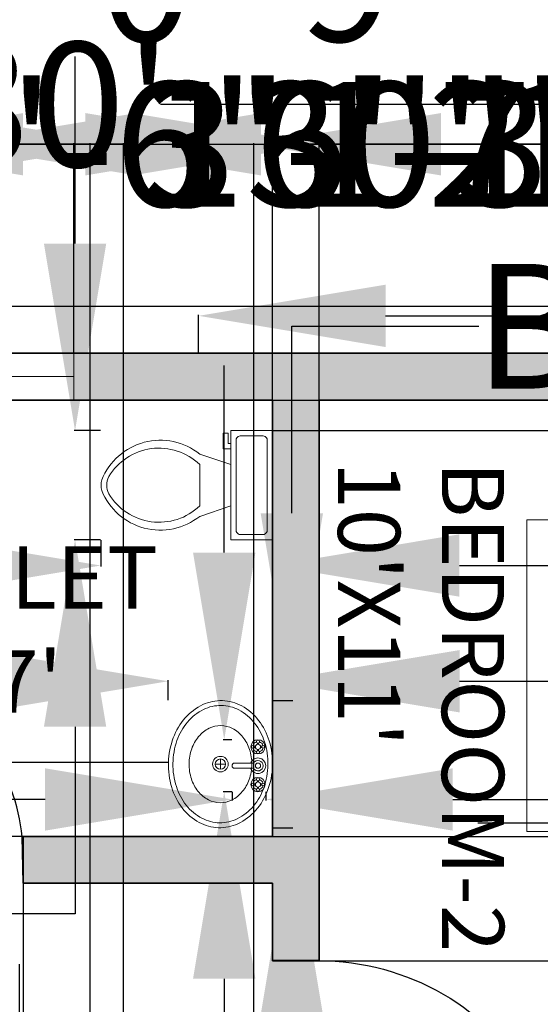
# Model space of a CAD drawing. Units: inches. Extents: x 2838 to 4029, y 1041 to 1915.
# Tile 12 of 16: x 3441 to 3541, y 1546 to 1735. Entities that reach past the tile are written whole.
import ezdxf

# ---------------------------------------------------------------- set-up
doc = ezdxf.new("R2010")
doc.units = ezdxf.units.IN
doc.header["$MEASUREMENT"] = 0
for name, color, linetype, lineweight in [('A-ANNO-DIMS', 2, 'Continuous', 18), ('A-AREA-IDEN', 7, 'Continuous', 18), ('A-DOOR', 3, 'Continuous', 25), ('A-FLOR', 7, 'Continuous', 25), ('A-FLOR-FIXT', 9, 'Continuous', 18), ('A-FURN', 8, 'Continuous', 18), ('A-GLAZ', 4, 'Continuous', 18), ('A-WALL', 7, 'Continuous', 35), ('A-WALL-PATT', 252, 'Continuous', 13)]:
    doc.layers.add(name, color=color, linetype=linetype, lineweight=lineweight)
doc.styles.get("Standard").update_dxf_attribs({"font": 'arial.ttf'})
doc.dimstyles.get("Standard").update_dxf_attribs({"dimtxt": 24, "dimasz": 36, "dimexe": 0.18, "dimexo": 0.0625, "dimgap": 0.09, "dimtad": 0, "dimtih": 1, "dimtoh": 1, "dimdec": 0, "dimzin": 0, "dimdsep": 46, "dimlunit": 3, "dimtxsty": 'Standard', "dimcen": 0.09, "dimadec": 0, "dimazin": 0, "dimtfac": 1, "dimtdec": 0, "dimtofl": 0, "dimtmove": 0, "dimatfit": 3, "dimfxl": 1, "dimtolj": 1, "dimtzin": 0, "dimarcsym": 0})

# ---------------------------------------------------------------- blocks, each defined once
blk = doc.blocks.new('*U2')
for p, q in [((0, 0), (0, -6)), ((40, 0), (40, -6))]:
    blk.add_line(p, q)
blk.add_lwpolyline([(0, 0), (34.64, 20), (35.52, 18.48), (0.87, -1.52)], close=True)
blk.add_arc((0, 0), 40, 0, 30)
blk = doc.blocks.new('*U3')
for p, q in [((-40, 0), (-40, 6)), ((0, 0), (0, 6))]:
    blk.add_line(p, q)
blk.add_lwpolyline([(0, 0), (-20, -34.64), (-21.52, -33.77), (-1.52, 0.88)], close=True)
blk.add_arc((0, 0), 40, 180, 240)
blk = doc.blocks.new('Toilet - top')
for p, q in [((9.5, -6), (9.5, -2)), ((-10, -8.5), (-8, -8.5)), ((-10, -9.5), (-10, -8.5)), ((-8, -8.5), (-8, -8)), ((-7, -8), (-7, -9.5)), ((-4, -8), (-6, -14)), ((4, -8), (6, -14)), ((-7, -9.5), (-10, -9.5)), ((4, -14), (-4, -14))]:
    blk.add_line(p, q)
blk.add_lwpolyline([(10.5, -8), (10.5, 0), (-10.5, 0), (-10.5, -8)], close=True)
for points in [[(8.5, -1), (-8.5, -1)], [(-9.5, -2), (-9.5, -6)], [(-8.5, -7), (8.5, -7)]]:
    blk.add_lwpolyline(points)
for centre, radius, start, end in [((-8.62, -1.88), 0.884, 81.8699, 188.1301), ((8.62, -1.88), 0.884, 351.8699, 98.1301), ((-8.62, -6.12), 0.884, 171.8699, 278.1301), ((8.62, -6.12), 0.884, 261.8699, 8.1301), ((3.52, -21.58), 12.17, 141.4691, 247.9714), ((4.2, -21.82), 11.33, 136.3677, 238.9468), ((-3.52, -21.58), 12.17, 292.0284, 38.5307), ((-4.2, -21.82), 11.33, 301.053, 43.6321), ((0, -27.88), 4, 245.7318, 294.2682), ((0, -29), 4, 254.8605, 285.1395)]:
    blk.add_arc(centre, radius, start, end)
blk = doc.blocks.new('Sink - Oval top')
for p, q in [((-1, 0), (1, 0)), ((0, 1), (0, -1))]:
    blk.add_line(p, q)
for points in [[(-12.23, 0.39, 0.117634), (-11.46, -3.36, 0.104469), (-8.88, -6.8, 0.090016), (-5.08, -9.07, 0.08192), (-0.32, -10.02, 0.08192), (4.49, -9.38, 0.090016), (8.42, -7.36, 0.104469), (11.22, -4.09, 0.117634), (12.23, -0.39, 0.117634), (11.46, 3.36, 0.104469), (8.88, 6.8, 0.090016), (5.08, 9.07, 0.08192), (0.32, 10.02, 0.08192), (-4.49, 9.38, 0.090016), (-8.42, 7.36, 0.104469), (-11.22, 4.09, 0.117634)], [(-11.29, 0.16, 0.118622), (-10.52, -3.25, 0.104678), (-8.07, -6.36, 0.089562), (-4.54, -8.37, 0.081185), (-0.13, -9.15, 0.081185), (4.3, -8.49, 0.089562), (7.89, -6.58, 0.104678), (10.42, -3.55, 0.118622), (11.29, -0.16, 0.118622), (10.52, 3.25, 0.104678), (8.07, 6.36, 0.089562), (4.54, 8.37, 0.081185), (0.13, 9.15, 0.081185), (-4.3, 8.49, 0.089562), (-7.89, 6.58, 0.104678), (-10.42, 3.55, 0.118622)], [(-7.42, 0.08, 0.118283), (-6.91, -2.17, 0.104607), (-5.29, -4.21, 0.089718), (-2.97, -5.53, 0.081436), (-0.07, -6.04, 0.081436), (2.84, -5.59, 0.089718), (5.2, -4.33, 0.104607), (6.86, -2.32, 0.118283), (7.42, -0.08, 0.118283), (6.91, 2.17, 0.104607), (5.29, 4.21, 0.089718), (2.97, 5.53, 0.081436), (0.07, 6.04, 0.081436), (-2.84, 5.59, 0.089718), (-5.2, 4.33, 0.104607), (-6.86, 2.32, 0.118283)]]:
    blk.add_lwpolyline(points, format="xyb", close=True)
for radius in [1.5, 1]:
    blk.add_circle((0, 0), radius)
blk = doc.blocks.new('Bed - Queen')
for p, q in [((0, -80.00003), (0, 0)), ((0, 0), (59.99999, 0)), ((59.99999, 0), (59.99999, -80.00003)), ((7.99999, -1.2), (28.79998, -1.2)), ((7.99999, -14.4), (7.99999, -1.2)), ((28.79998, -1.2), (28.79998, -14.4)), ((31.19999, -1.2), (51.99999, -1.2)), ((31.19999, -14.4), (31.19999, -1.2)), ((51.99999, -1.2), (51.99999, -16.4)), ((0, -14.4), (44.8, -14.4)), ((59.99999, -29.6), (44.8, -14.4)), ((44.8, -14.4), (44.8, -29.6)), ((44.8, -16.8), (0, -16.8)), ((51.99999, -16.4), (46.79936, -16.4)), ((44.8, -29.6), (59.99999, -29.6)), ((59.99999, -80.00003), (0, -80.00003))]:
    blk.add_line(p, q)
blk = doc.blocks.new('Faucet - Bathroom top')
for p, q in [((-4.107, 0.125), (-4.375, 0.125)), ((-3.75, 0.4788), (-3.75, 0.75)), ((-3.5, 0.482), (-3.5, 0.75)), ((-3.1461, 0.125), (-2.875, 0.125)), ((3.143, 0.125), (2.875, 0.125)), ((3.5, 0.4788), (3.5, 0.75)), ((3.75, 0.482), (3.75, 0.75)), ((4.1039, 0.125), (4.375, 0.125)), ((-4.1039, -0.125), (-4.375, -0.125)), ((-3.75, -0.4821), (-3.75, -0.75)), ((-3.5, -0.4789), (-3.5, -0.75)), ((-3.143, -0.125), (-2.875, -0.125)), ((-0.5, -0.8639), (-0.5, -4.5)), ((0.5, -4.5), (0.5, -0.8631)), ((3.1461, -0.125), (2.875, -0.125)), ((3.5, -0.4821), (3.5, -0.75)), ((3.75, -0.4789), (3.75, -0.75)), ((4.107, -0.125), (4.375, -0.125))]:
    blk.add_line(p, q)
for centre, radius in [((-3.625, 0), 1.375), ((-4.625, 0), 0.2795), ((-3.625, 0), 0.5), ((-3.625, 1), 0.2795), ((-2.625, 0), 0.2795), ((0, 0), 0.5), ((3.625, 0), 1.375), ((2.625, 0), 0.2795), ((3.625, 0), 0.5), ((3.625, 1), 0.2795), ((4.625, 0), 0.2795), ((-3.625, -1), 0.2795), ((3.625, -1), 0.2795)]:
    blk.add_circle(centre, radius)
for centre, radius, start, end in [((-3.625, 0), 1, 105.2407, 164.2093), ((-3.625, 0), 1, 16.44125, 74.07887), ((0, 0), 1.5, 289.6514, 250.3603), ((0, 0), 1, 300.3431, 239.7554), ((3.625, 0), 1, 106.12, 164.0884), ((3.625, 0), 1, 16.23422, 73.90469), ((-3.625, 0), 1, 196.2342, 253.9047), ((-3.625, 0), 1, 286.12, 344.0884), ((3.625, 0), 1, 196.4413, 254.0789), ((3.625, 0), 1, 285.2407, 344.2093), ((0, -4.5), 0.5, 180, 0)]:
    blk.add_arc(centre, radius, start, end)
blk = doc.blocks.new('*D18')
at = {"layer": 'A-ANNO-DIMS', "color": 0, "lineweight": -2, "transparency": 16777216}
for p, q in [((3267.73, 1671.36), (3267.73, 1719.35)), ((3303.73, 1719.17), (3427.28, 1719.17)), ((3591.73, 1719.17), (3468.18, 1719.17)), ((3627.73, 1671.36), (3627.73, 1719.35))]:
    blk.add_line(p, q, dxfattribs=at)
at = {"layer": 'A-ANNO-DIMS', "color": 0, "transparency": 16777216}
for points in [[(3303.73, 1725.17), (3303.73, 1713.17), (3267.73, 1719.17)], [(3591.73, 1725.17), (3591.73, 1713.17), (3627.73, 1719.17)]]:
    blk.add_solid(points, dxfattribs=at)
at = {"layer": 'Defpoints', "color": 0, "transparency": 16777216}
for p in [(3267.73, 1719.17), (3267.73, 1671.3), (3627.73, 1671.3)]:
    blk.add_point(p, dxfattribs=at)
at = {"layer": 'A-ANNO-DIMS', "color": 0, "transparency": 16777216, "insert": (3447.73, 1719.17), "char_height": 24, "attachment_point": 5}
blk.add_mtext("\\A1;30'", dxfattribs=at)
blk = doc.blocks.new('WIN-24-VENT')
for p, q in [((24, 9), (24, 0)), ((24, 4.5), (0, 4.5))]:
    blk.add_line(p, q)
blk.add_lwpolyline([(48, 0), (0, 0), (0, 9), (48, 9)])
blk = doc.blocks.new('*D28')
at = {"layer": 'A-ANNO-DIMS', "color": 0, "lineweight": -2, "transparency": 16777216}
for p, q in [((3565.25, 1580.88), (3529.25, 1580.88)), ((3601.25, 1578.37), (3601.25, 1581.06)), ((3617.82, 1578.37), (3617.82, 1581.06)), ((3653.82, 1580.88), (3689.82, 1580.88))]:
    blk.add_line(p, q, dxfattribs=at)
at = {"layer": 'A-ANNO-DIMS', "color": 0, "transparency": 16777216}
for points in [[(3565.25, 1586.88), (3565.25, 1574.88), (3601.25, 1580.88)], [(3653.82, 1586.88), (3653.82, 1574.88), (3617.82, 1580.88)]]:
    blk.add_solid(points, dxfattribs=at)
at = {"layer": 'Defpoints', "color": 0, "transparency": 16777216}
for p in [(3617.82, 1580.88), (3601.25, 1578.31), (3617.82, 1578.31)]:
    blk.add_point(p, dxfattribs=at)
at = {"layer": 'A-ANNO-DIMS', "color": 0, "transparency": 16777216, "insert": (3789.89, 1580.88), "char_height": 24, "attachment_point": 5}
blk.add_mtext('\\A1;1\'-4 1/2" TYP.', dxfattribs=at)
blk = doc.blocks.new('*D35')
at = {"layer": 'A-ANNO-DIMS', "color": 0, "lineweight": -2, "transparency": 16777216}
for p, q in [((3480.45, 1632.93), (3480.45, 1668.93)), ((3481.89, 1596.93), (3480.27, 1596.93)), ((3481.89, 1586.93), (3480.27, 1586.93)), ((3480.45, 1550.93), (3480.45, 1514.93)), ((3480.45, 1514.93), (3444.45, 1514.93))]:
    blk.add_line(p, q, dxfattribs=at)
at = {"layer": 'A-ANNO-DIMS', "color": 0, "transparency": 16777216}
for points in [[(3474.45, 1632.93), (3486.45, 1632.93), (3480.45, 1596.93)], [(3474.45, 1550.93), (3486.45, 1550.93), (3480.45, 1586.93)]]:
    blk.add_solid(points, dxfattribs=at)
at = {"layer": 'Defpoints', "color": 0, "transparency": 16777216}
for p in [(3481.95, 1596.93), (3480.45, 1586.93), (3481.95, 1586.93)]:
    blk.add_point(p, dxfattribs=at)
at = {"layer": 'A-ANNO-DIMS', "color": 0, "transparency": 16777216, "insert": (3365.58, 1514.93), "char_height": 24, "attachment_point": 5}
blk.add_mtext('\\A1;TAP 0\'-10"', dxfattribs=at)
blk = doc.blocks.new('*D36')
at = {"layer": 'A-ANNO-DIMS', "color": 0, "lineweight": -2, "transparency": 16777216}
for p, q in [((3481.95, 1586.87), (3481.95, 1585.25)), ((3488.45, 1586.87), (3488.45, 1585.25)), ((3445.95, 1585.43), (3409.95, 1585.43)), ((3524.45, 1585.43), (3560.45, 1585.43))]:
    blk.add_line(p, q, dxfattribs=at)
at = {"layer": 'A-ANNO-DIMS', "color": 0, "transparency": 16777216}
for points in [[(3445.95, 1591.43), (3445.95, 1579.43), (3481.95, 1585.43)], [(3524.45, 1591.43), (3524.45, 1579.43), (3488.45, 1585.43)]]:
    blk.add_solid(points, dxfattribs=at)
at = {"layer": 'Defpoints', "color": 0, "transparency": 16777216}
for p in [(3481.95, 1586.93), (3488.45, 1586.93), (3488.45, 1585.43)]:
    blk.add_point(p, dxfattribs=at)
at = {"layer": 'A-ANNO-DIMS', "color": 0, "transparency": 16777216, "insert": (3620.4, 1585.43), "char_height": 24, "attachment_point": 5}
blk.add_mtext('\\A1;0\'-6 1/2"', dxfattribs=at)
blk = doc.blocks.new('*D39')
at = {"layer": 'A-ANNO-DIMS', "color": 0, "lineweight": -2, "transparency": 16777216}
for p, q in [((3391.52, 1678.5), (3355.52, 1678.5)), ((3427.52, 1671.36), (3427.52, 1678.68)), ((3475.52, 1671.36), (3475.52, 1678.68)), ((3511.52, 1678.5), (3547.52, 1678.5))]:
    blk.add_line(p, q, dxfattribs=at)
at = {"layer": 'A-ANNO-DIMS', "color": 0, "transparency": 16777216}
for points in [[(3391.52, 1684.5), (3391.52, 1672.5), (3427.52, 1678.5)], [(3511.52, 1684.5), (3511.52, 1672.5), (3475.52, 1678.5)]]:
    blk.add_solid(points, dxfattribs=at)
at = {"layer": 'Defpoints', "color": 0, "transparency": 16777216}
for p in [(3475.52, 1678.5), (3427.52, 1671.3), (3475.52, 1671.3)]:
    blk.add_point(p, dxfattribs=at)
at = {"layer": 'A-ANNO-DIMS', "color": 0, "transparency": 16777216, "insert": (3732.24, 1678.5), "char_height": 24, "attachment_point": 5}
blk.add_mtext('\\A1;VENT BLOCK 4\'-0" TYP.', dxfattribs=at)
blk = doc.blocks.new('*D40')
at = {"layer": 'A-ANNO-DIMS', "color": 0, "lineweight": -2, "transparency": 16777216}
for p, q in [((3420.32, 1707.3), (3420.32, 1743.3)), ((3420.32, 1743.3), (3456.32, 1743.3)), ((3427.46, 1671.3), (3420.14, 1671.3)), ((3427.46, 1662.3), (3420.14, 1662.3)), ((3420.32, 1626.3), (3420.32, 1590.3))]:
    blk.add_line(p, q, dxfattribs=at)
at = {"layer": 'A-ANNO-DIMS', "color": 0, "transparency": 16777216}
for points in [[(3414.32, 1707.3), (3426.32, 1707.3), (3420.32, 1671.3)], [(3414.32, 1626.3), (3426.32, 1626.3), (3420.32, 1662.3)]]:
    blk.add_solid(points, dxfattribs=at)
at = {"layer": 'Defpoints', "color": 0, "transparency": 16777216}
for p in [(3420.32, 1671.3), (3427.52, 1671.3), (3427.52, 1662.3)]:
    blk.add_point(p, dxfattribs=at)
at = {"layer": 'A-ANNO-DIMS', "color": 0, "transparency": 16777216, "insert": (3529.56, 1743.3), "char_height": 24, "attachment_point": 5}
blk.add_mtext('\\A1;0\'-9" TYP.', dxfattribs=at)
blk = doc.blocks.new('*D41')
at = {"layer": 'A-ANNO-DIMS', "color": 0, "lineweight": -2, "transparency": 16777216}
for p, q in [((3284.24, 1506.2), (3284.24, 1496.56)), ((3347.73, 1506.2), (3347.73, 1496.56)), ((3248.24, 1496.74), (3212.24, 1496.74)), ((3383.73, 1496.74), (3419.73, 1496.74))]:
    blk.add_line(p, q, dxfattribs=at)
at = {"layer": 'A-ANNO-DIMS', "color": 0, "transparency": 16777216}
for points in [[(3248.24, 1502.74), (3248.24, 1490.74), (3284.24, 1496.74)], [(3383.73, 1502.74), (3383.73, 1490.74), (3347.73, 1496.74)]]:
    blk.add_solid(points, dxfattribs=at)
at = {"layer": 'Defpoints', "color": 0, "transparency": 16777216}
for p in [(3284.24, 1506.26), (3347.73, 1506.26), (3347.73, 1496.74)]:
    blk.add_point(p, dxfattribs=at)
at = {"layer": 'A-ANNO-DIMS', "color": 0, "transparency": 16777216, "insert": (3624.81, 1496.74), "char_height": 24, "attachment_point": 5}
blk.add_mtext('\\A1;WARDROBE 5\'-3 1/2" TYP.', dxfattribs=at)
blk = doc.blocks.new('*D45')
at = {"layer": 'A-ANNO-DIMS', "color": 0, "lineweight": -2, "transparency": 16777216}
for p, q in [((3456.69, 1635.35), (3456.69, 1630.27)), ((3489.73, 1635.35), (3489.73, 1630.27)), ((3420.69, 1630.45), (3384.69, 1630.45)), ((3525.73, 1630.45), (3561.73, 1630.45))]:
    blk.add_line(p, q, dxfattribs=at)
at = {"layer": 'A-ANNO-DIMS', "color": 0, "transparency": 16777216}
for points in [[(3420.69, 1636.45), (3420.69, 1624.45), (3456.69, 1630.45)], [(3525.73, 1636.45), (3525.73, 1624.45), (3489.73, 1630.45)]]:
    blk.add_solid(points, dxfattribs=at)
at = {"layer": 'Defpoints', "color": 0, "transparency": 16777216}
for p in [(3456.69, 1635.41), (3489.73, 1635.41), (3489.73, 1630.45)]:
    blk.add_point(p, dxfattribs=at)
at = {"layer": 'A-ANNO-DIMS', "color": 0, "transparency": 16777216, "insert": (3626.8, 1630.45), "char_height": 24, "attachment_point": 5}
blk.add_mtext('\\A1;WC 2\'-9"', dxfattribs=at)
blk = doc.blocks.new('*D46')
at = {"layer": 'A-ANNO-DIMS', "color": 0, "lineweight": -2, "transparency": 16777216}
for p, q in [((3451.73, 1692.41), (3451.73, 1728.41)), ((3456.62, 1656.41), (3451.55, 1656.41)), ((3456.62, 1635.41), (3451.55, 1635.41)), ((3451.73, 1599.41), (3451.73, 1563.41)), ((3451.73, 1563.41), (3415.73, 1563.41))]:
    blk.add_line(p, q, dxfattribs=at)
at = {"layer": 'A-ANNO-DIMS', "color": 0, "transparency": 16777216}
for points in [[(3445.73, 1692.41), (3457.73, 1692.41), (3451.73, 1656.41)], [(3445.73, 1599.41), (3457.73, 1599.41), (3451.73, 1635.41)]]:
    blk.add_solid(points, dxfattribs=at)
at = {"layer": 'Defpoints', "color": 0, "transparency": 16777216}
for p in [(3456.69, 1656.41), (3451.73, 1635.41), (3456.69, 1635.41)]:
    blk.add_point(p, dxfattribs=at)
at = {"layer": 'A-ANNO-DIMS', "color": 0, "transparency": 16777216, "insert": (3384.87, 1563.41), "char_height": 24, "attachment_point": 5}
blk.add_mtext('\\A1;1\'-9"', dxfattribs=at)
blk = doc.blocks.new('*D47')
at = {"layer": 'A-ANNO-DIMS', "color": 0, "lineweight": -2, "transparency": 16777216}
for p, q in [((3493.47, 1640.5), (3493.47, 1676.5)), ((3493.47, 1676.5), (3529.47, 1676.5)), ((3489.85, 1604.5), (3493.65, 1604.5)), ((3489.85, 1579.95), (3493.65, 1579.95)), ((3493.47, 1543.95), (3493.47, 1507.95))]:
    blk.add_line(p, q, dxfattribs=at)
at = {"layer": 'A-ANNO-DIMS', "color": 0, "transparency": 16777216}
for points in [[(3487.47, 1640.5), (3499.47, 1640.5), (3493.47, 1604.5)], [(3487.47, 1543.95), (3499.47, 1543.95), (3493.47, 1579.95)]]:
    blk.add_solid(points, dxfattribs=at)
at = {"layer": 'Defpoints', "color": 0, "transparency": 16777216}
for p in [(3489.78, 1604.5), (3493.47, 1604.5), (3489.78, 1579.95)]:
    blk.add_point(p, dxfattribs=at)
at = {"layer": 'A-ANNO-DIMS', "color": 0, "transparency": 16777216, "insert": (3643.85, 1676.5), "char_height": 24, "attachment_point": 5}
blk.add_mtext('\\A1;BASIN 2\'-0 1/2"', dxfattribs=at)
blk = doc.blocks.new('*D48')
at = {"layer": 'A-ANNO-DIMS', "color": 0, "lineweight": -2, "transparency": 16777216}
for p, q in [((3433.65, 1608.18), (3397.65, 1608.18)), ((3469.65, 1604.56), (3469.65, 1608.36)), ((3489.78, 1604.56), (3489.78, 1608.36)), ((3525.78, 1608.18), (3561.78, 1608.18))]:
    blk.add_line(p, q, dxfattribs=at)
at = {"layer": 'A-ANNO-DIMS', "color": 0, "transparency": 16777216}
for points in [[(3433.65, 1614.18), (3433.65, 1602.18), (3469.65, 1608.18)], [(3525.78, 1614.18), (3525.78, 1602.18), (3489.78, 1608.18)]]:
    blk.add_solid(points, dxfattribs=at)
at = {"layer": 'Defpoints', "color": 0, "transparency": 16777216}
for p in [(3469.65, 1608.18), (3469.65, 1604.5), (3489.78, 1604.5)]:
    blk.add_point(p, dxfattribs=at)
at = {"layer": 'A-ANNO-DIMS', "color": 0, "transparency": 16777216, "insert": (3366.79, 1608.18), "char_height": 24, "attachment_point": 5}
blk.add_mtext('\\A1;1\'-8"', dxfattribs=at)
blk = doc.blocks.new('*D50')
at = {"layer": 'A-ANNO-DIMS', "color": 0, "lineweight": -2, "transparency": 16777216}
for p, q in [((3441.02, 1517.75), (3441.02, 1553.75)), ((3427.44, 1481.75), (3441.2, 1481.75)), ((3427.44, 1426.75), (3441.2, 1426.75)), ((3441.02, 1390.75), (3441.02, 1354.75))]:
    blk.add_line(p, q, dxfattribs=at)
at = {"layer": 'A-ANNO-DIMS', "color": 0, "transparency": 16777216}
for points in [[(3435.02, 1517.75), (3447.02, 1517.75), (3441.02, 1481.75)], [(3435.02, 1390.75), (3447.02, 1390.75), (3441.02, 1426.75)]]:
    blk.add_solid(points, dxfattribs=at)
at = {"layer": 'Defpoints', "color": 0, "transparency": 16777216}
for p in [(3427.37, 1481.75), (3441.02, 1481.75), (3427.37, 1426.75)]:
    blk.add_point(p, dxfattribs=at)
at = {"layer": 'A-ANNO-DIMS', "color": 0, "transparency": 16777216, "insert": (3441.02, 1454.25), "char_height": 24, "attachment_point": 5}
blk.add_mtext('\\A1;4\'-7"', dxfattribs=at)
blk = doc.blocks.new('*D55')
at = {"layer": 'A-ANNO-DIMS', "color": 0, "lineweight": -2, "transparency": 16777216}
for p, q in [((3491.76, 1499.78), (3455.76, 1499.78)), ((3527.76, 1494.67), (3527.76, 1499.96)), ((3562.26, 1494.67), (3562.26, 1499.96)), ((3598.26, 1499.78), (3634.26, 1499.78))]:
    blk.add_line(p, q, dxfattribs=at)
at = {"layer": 'A-ANNO-DIMS', "color": 0, "transparency": 16777216}
for points in [[(3491.76, 1505.78), (3491.76, 1493.78), (3527.76, 1499.78)], [(3598.26, 1505.78), (3598.26, 1493.78), (3562.26, 1499.78)]]:
    blk.add_solid(points, dxfattribs=at)
at = {"layer": 'Defpoints', "color": 0, "transparency": 16777216}
for p in [(3527.76, 1499.78), (3527.76, 1494.6), (3562.26, 1494.6)]:
    blk.add_point(p, dxfattribs=at)
at = {"layer": 'A-ANNO-DIMS', "color": 0, "transparency": 16777216, "insert": (3260.33, 1499.78), "char_height": 24, "attachment_point": 5}
blk.add_mtext('\\A1;BASE CABINET 2\'-10 1/2"', dxfattribs=at)
blk = doc.blocks.new('*D68')
at = {"layer": 'A-ANNO-DIMS', "color": 0, "lineweight": -2, "transparency": 16777216}
for p, q in [((3258.73, 1680.36), (3258.73, 1711.7)), ((3294.73, 1711.52), (3406.43, 1711.52)), ((3600.73, 1711.52), (3489.04, 1711.52)), ((3636.73, 1680.36), (3636.73, 1711.7))]:
    blk.add_line(p, q, dxfattribs=at)
at = {"layer": 'A-ANNO-DIMS', "color": 0, "transparency": 16777216}
for points in [[(3294.73, 1717.52), (3294.73, 1705.52), (3258.73, 1711.52)], [(3600.73, 1717.52), (3600.73, 1705.52), (3636.73, 1711.52)]]:
    blk.add_solid(points, dxfattribs=at)
at = {"layer": 'Defpoints', "color": 0, "transparency": 16777216}
for p in [(3636.73, 1711.52), (3258.73, 1680.3), (3636.73, 1680.3)]:
    blk.add_point(p, dxfattribs=at)
at = {"layer": 'A-ANNO-DIMS', "color": 0, "transparency": 16777216, "insert": (3447.73, 1711.52), "char_height": 24, "attachment_point": 5}
blk.add_mtext('\\A1;31\'-6"', dxfattribs=at)
blk = doc.blocks.new('*D73')
at = {"layer": 'A-ANNO-DIMS', "color": 0, "lineweight": -2, "transparency": 16777216}
for p, q in [((3425.038746, 1711.522346), (3389.038746, 1711.522346)), ((3461.038746, 1200.359846), (3461.038746, 1711.702346)), ((3618.731626, 1200.359846), (3618.731626, 1711.702346)), ((3654.731626, 1711.522346), (3690.731626, 1711.522346))]:
    blk.add_line(p, q, dxfattribs=at)
at = {"layer": 'A-ANNO-DIMS', "color": 0, "transparency": 16777216}
for points in [[(3425.038746, 1717.522346), (3425.038746, 1705.522346), (3461.038746, 1711.522346)], [(3654.731626, 1717.522346), (3654.731626, 1705.522346), (3618.731626, 1711.522346)]]:
    blk.add_solid(points, dxfattribs=at)
at = {"layer": 'Defpoints', "color": 0, "transparency": 16777216}
for p in [(3618.731626, 1711.522346), (3461.038746, 1200.297346), (3618.731626, 1200.297346)]:
    blk.add_point(p, dxfattribs=at)
at = {"layer": 'A-ANNO-DIMS', "color": 0, "transparency": 16777216, "insert": (3539.885186, 1711.522346), "char_height": 24, "attachment_point": 5}
blk.add_mtext('\\A1;13\'-1 1/2"', dxfattribs=at)
blk = doc.blocks.new('*D78')
at = {"layer": 'A-ANNO-DIMS', "color": 0, "lineweight": -2, "transparency": 16777216}
for p, q in [((3667.956626, 1590.394218), (3667.956626, 1626.394218)), ((3498.794126, 1554.394218), (3668.136626, 1554.394218)), ((3498.638013, 1506.394218), (3668.136626, 1506.394218)), ((3667.956626, 1470.394218), (3667.956626, 1434.394218))]:
    blk.add_line(p, q, dxfattribs=at)
at = {"layer": 'A-ANNO-DIMS', "color": 0, "transparency": 16777216}
for points in [[(3661.956626, 1590.394218), (3673.956626, 1590.394218), (3667.956626, 1554.394218)], [(3661.956626, 1470.394218), (3673.956626, 1470.394218), (3667.956626, 1506.394218)]]:
    blk.add_solid(points, dxfattribs=at)
at = {"layer": 'Defpoints', "color": 0, "transparency": 16777216}
for p in [(3498.731626, 1554.394218), (3667.956626, 1554.394218), (3498.575513, 1506.394218)]:
    blk.add_point(p, dxfattribs=at)
at = {"layer": 'A-ANNO-DIMS', "color": 0, "transparency": 16777216, "insert": (3667.956626, 1530.394218), "char_height": 24, "attachment_point": 5}
blk.add_mtext('\\A1;4\'-0"', dxfattribs=at)
blk = doc.blocks.new('*D79')
at = {"layer": 'A-ANNO-DIMS', "color": 0, "lineweight": -2, "transparency": 16777216}
for p, q in [((3379.05, 1400.64), (3379.05, 1711.7)), ((3415.05, 1711.52), (3418.63, 1711.52)), ((3454.63, 1398.31), (3454.63, 1711.7)), ((3454.63, 1711.52), (3490.63, 1711.52))]:
    blk.add_line(p, q, dxfattribs=at)
at = {"layer": 'A-ANNO-DIMS', "color": 0, "transparency": 16777216}
for points in [[(3415.05, 1717.52), (3415.05, 1705.52), (3379.05, 1711.52)], [(3418.63, 1717.52), (3418.63, 1705.52), (3454.63, 1711.52)]]:
    blk.add_solid(points, dxfattribs=at)
at = {"layer": 'Defpoints', "color": 0, "transparency": 16777216}
for p in [(3454.63, 1711.52), (3379.05, 1400.57), (3454.63, 1398.25)]:
    blk.add_point(p, dxfattribs=at)
at = {"layer": 'A-ANNO-DIMS', "color": 0, "transparency": 16777216, "insert": (3550.65, 1711.52), "char_height": 24, "attachment_point": 5}
blk.add_mtext('\\A1;6\'-3 1/2"', dxfattribs=at)
blk = doc.blocks.new('*D80')
at = {"layer": 'A-ANNO-DIMS', "color": 0, "lineweight": -2, "transparency": 16777216}
for p, q in [((3324.91, 1711.52), (3288.91, 1711.52)), ((3360.91, 1662.36), (3360.91, 1711.7)), ((3396.73, 1662.36), (3396.73, 1711.7)), ((3432.73, 1711.52), (3468.73, 1711.52))]:
    blk.add_line(p, q, dxfattribs=at)
at = {"layer": 'A-ANNO-DIMS', "color": 0, "transparency": 16777216}
for points in [[(3324.91, 1717.52), (3324.91, 1705.52), (3360.91, 1711.52)], [(3432.73, 1717.52), (3432.73, 1705.52), (3396.73, 1711.52)]]:
    blk.add_solid(points, dxfattribs=at)
at = {"layer": 'Defpoints', "color": 0, "transparency": 16777216}
for p in [(3396.73, 1711.52), (3360.91, 1662.3), (3396.73, 1662.3)]:
    blk.add_point(p, dxfattribs=at)
at = {"layer": 'A-ANNO-DIMS', "color": 0, "transparency": 16777216, "insert": (3500.71, 1711.52), "char_height": 24, "attachment_point": 5}
blk.add_mtext('\\A1;3\'-0"', dxfattribs=at)
blk = doc.blocks.new('*D82')
at = {"layer": 'A-ANNO-DIMS', "color": 0, "lineweight": -2, "transparency": 16777216}
for p, q in [((3405.73, 1573.06), (3405.73, 1081.89)), ((3441.73, 1569.23), (3441.73, 1081.89)), ((3369.73, 1082.07), (3333.73, 1082.07)), ((3477.73, 1082.07), (3513.73, 1082.07))]:
    blk.add_line(p, q, dxfattribs=at)
at = {"layer": 'A-ANNO-DIMS', "color": 0, "transparency": 16777216}
for points in [[(3369.73, 1088.07), (3369.73, 1076.07), (3405.73, 1082.07)], [(3477.73, 1088.07), (3477.73, 1076.07), (3441.73, 1082.07)]]:
    blk.add_solid(points, dxfattribs=at)
at = {"layer": 'Defpoints', "color": 0, "transparency": 16777216}
for p in [(3405.73, 1573.12), (3441.73, 1569.3), (3441.73, 1082.07)]:
    blk.add_point(p, dxfattribs=at)
at = {"layer": 'A-ANNO-DIMS', "color": 0, "transparency": 16777216, "insert": (3545.71, 1082.07), "char_height": 24, "attachment_point": 5}
blk.add_mtext('\\A1;3\'-0"', dxfattribs=at)
blk = doc.blocks.new('*D83')
at = {"layer": 'A-ANNO-DIMS', "color": 0, "lineweight": -2, "transparency": 16777216}
for p, q in [((3405.73, 1662.36), (3405.73, 1711.7)), ((3441.73, 1711.52), (3453.73, 1711.52)), ((3489.73, 1662.36), (3489.73, 1711.7)), ((3489.73, 1711.52), (3525.73, 1711.52))]:
    blk.add_line(p, q, dxfattribs=at)
at = {"layer": 'A-ANNO-DIMS', "color": 0, "transparency": 16777216}
for points in [[(3441.73, 1717.52), (3441.73, 1705.52), (3405.73, 1711.52)], [(3453.73, 1717.52), (3453.73, 1705.52), (3489.73, 1711.52)]]:
    blk.add_solid(points, dxfattribs=at)
at = {"layer": 'Defpoints', "color": 0, "transparency": 16777216}
for p in [(3489.73, 1711.52), (3405.73, 1662.3), (3489.73, 1662.3)]:
    blk.add_point(p, dxfattribs=at)
at = {"layer": 'A-ANNO-DIMS', "color": 0, "transparency": 16777216, "insert": (3557.62, 1711.52), "char_height": 24, "attachment_point": 5}
blk.add_mtext('\\A1;7\'-0"', dxfattribs=at)
blk = doc.blocks.new('*D84')
at = {"layer": 'A-ANNO-DIMS', "color": 0, "lineweight": -2, "transparency": 16777216}
for p, q in [((3667.96, 1662.3), (3667.96, 1698.3)), ((3667.96, 1698.3), (3703.96, 1698.3)), ((3489.79, 1662.3), (3668.14, 1662.3)), ((3667.96, 1614.3), (3667.96, 1626.3)), ((3489.79, 1578.3), (3668.14, 1578.3))]:
    blk.add_line(p, q, dxfattribs=at)
at = {"layer": 'A-ANNO-DIMS', "color": 0, "transparency": 16777216}
for points in [[(3661.96, 1626.3), (3673.96, 1626.3), (3667.96, 1662.3)], [(3661.96, 1614.3), (3673.96, 1614.3), (3667.96, 1578.3)]]:
    blk.add_solid(points, dxfattribs=at)
at = {"layer": 'Defpoints', "color": 0, "transparency": 16777216}
for p in [(3489.73, 1662.3), (3667.96, 1662.3), (3489.73, 1578.3)]:
    blk.add_point(p, dxfattribs=at)
at = {"layer": 'A-ANNO-DIMS', "color": 0, "transparency": 16777216, "insert": (3735.85, 1698.3), "char_height": 24, "attachment_point": 5}
blk.add_mtext('\\A1;7\'-0"', dxfattribs=at)
blk = doc.blocks.new('*D85')
at = {"layer": 'A-ANNO-DIMS', "color": 0, "lineweight": -2, "transparency": 16777216}
for p, q in [((3369.73, 1711.52), (3333.73, 1711.52)), ((3405.73, 1662.36), (3405.73, 1711.7)), ((3427.52, 1662.36), (3427.52, 1711.7)), ((3463.52, 1711.52), (3499.52, 1711.52))]:
    blk.add_line(p, q, dxfattribs=at)
at = {"layer": 'A-ANNO-DIMS', "color": 0, "transparency": 16777216}
for points in [[(3369.73, 1717.52), (3369.73, 1705.52), (3405.73, 1711.52)], [(3463.52, 1717.52), (3463.52, 1705.52), (3427.52, 1711.52)]]:
    blk.add_solid(points, dxfattribs=at)
at = {"layer": 'Defpoints', "color": 0, "transparency": 16777216}
for p in [(3427.52, 1711.52), (3405.73, 1662.3), (3427.52, 1662.3)]:
    blk.add_point(p, dxfattribs=at)
at = {"layer": 'A-ANNO-DIMS', "color": 0, "transparency": 16777216, "insert": (3539.7, 1711.52), "char_height": 24, "attachment_point": 5}
blk.add_mtext('\\A1;1\'-10"', dxfattribs=at)
blk = doc.blocks.new('*D86')
at = {"layer": 'A-ANNO-DIMS', "color": 0, "lineweight": -2, "transparency": 16777216}
for p, q in [((3391.52, 1711.52), (3355.52, 1711.52)), ((3427.52, 1671.36), (3427.52, 1711.7)), ((3451.52, 1671.36), (3451.52, 1711.7)), ((3487.52, 1711.52), (3523.52, 1711.52))]:
    blk.add_line(p, q, dxfattribs=at)
at = {"layer": 'A-ANNO-DIMS', "color": 0, "transparency": 16777216}
for points in [[(3391.52, 1717.52), (3391.52, 1705.52), (3427.52, 1711.52)], [(3487.52, 1717.52), (3487.52, 1705.52), (3451.52, 1711.52)]]:
    blk.add_solid(points, dxfattribs=at)
at = {"layer": 'Defpoints', "color": 0, "transparency": 16777216}
for p in [(3451.52, 1711.52), (3427.52, 1671.3), (3451.52, 1671.3)]:
    blk.add_point(p, dxfattribs=at)
at = {"layer": 'A-ANNO-DIMS', "color": 0, "transparency": 16777216, "insert": (3555.72, 1711.52), "char_height": 24, "attachment_point": 5}
blk.add_mtext('\\A1;2\'-0"', dxfattribs=at)
blk = doc.blocks.new('*D91')
at = {"layer": 'A-ANNO-DIMS', "color": 0, "lineweight": -2, "transparency": 16777216}
for p, q in [((3227.506626, 1533.394218), (3227.506626, 1569.394218)), ((3522.669126, 1497.394218), (3227.326626, 1497.394218)), ((3522.669126, 1461.394218), (3227.326626, 1461.394218)), ((3227.506626, 1425.394218), (3227.506626, 1389.394218))]:
    blk.add_line(p, q, dxfattribs=at)
at = {"layer": 'A-ANNO-DIMS', "color": 0, "transparency": 16777216}
for points in [[(3221.506626, 1533.394218), (3233.506626, 1533.394218), (3227.506626, 1497.394218)], [(3221.506626, 1425.394218), (3233.506626, 1425.394218), (3227.506626, 1461.394218)]]:
    blk.add_solid(points, dxfattribs=at)
at = {"layer": 'Defpoints', "color": 0, "transparency": 16777216}
for p in [(3522.731626, 1497.394218), (3227.506626, 1461.394218), (3522.731626, 1461.394218)]:
    blk.add_point(p, dxfattribs=at)
at = {"layer": 'A-ANNO-DIMS', "color": 0, "transparency": 16777216, "insert": (3227.506626, 1479.394218), "char_height": 24, "attachment_point": 5}
blk.add_mtext('\\A1;3\'-0"', dxfattribs=at)
blk = doc.blocks.new('*D96')
at = {"layer": 'A-ANNO-DIMS', "color": 0, "lineweight": -2, "transparency": 16777216}
for p, q in [((3462.73, 1711.52), (3426.73, 1711.52)), ((3498.73, 1662.36), (3498.73, 1711.7)), ((3546.42, 1662.36), (3546.42, 1711.7)), ((3582.42, 1711.52), (3618.42, 1711.52))]:
    blk.add_line(p, q, dxfattribs=at)
at = {"layer": 'A-ANNO-DIMS', "color": 0, "transparency": 16777216}
for points in [[(3462.73, 1717.52), (3462.73, 1705.52), (3498.73, 1711.52)], [(3582.42, 1717.52), (3582.42, 1705.52), (3546.42, 1711.52)]]:
    blk.add_solid(points, dxfattribs=at)
at = {"layer": 'Defpoints', "color": 0, "transparency": 16777216}
for p in [(3546.42, 1711.52), (3498.73, 1662.3), (3546.42, 1662.3)]:
    blk.add_point(p, dxfattribs=at)
at = {"layer": 'A-ANNO-DIMS', "color": 0, "transparency": 16777216, "insert": (3687.68, 1711.52), "char_height": 24, "attachment_point": 5}
blk.add_mtext('\\A1;3\'-11 1/2"', dxfattribs=at)
blk = doc.blocks.new('*D101')
at = {"layer": 'A-ANNO-DIMS', "color": 0, "lineweight": -2, "transparency": 16777216}
for p, q in [((3425.04, 1711.52), (3389.04, 1711.52)), ((3461.04, 1200.36), (3461.04, 1711.7)), ((3486.18, 1200.36), (3486.18, 1711.7)), ((3522.18, 1711.52), (3558.18, 1711.52))]:
    blk.add_line(p, q, dxfattribs=at)
at = {"layer": 'A-ANNO-DIMS', "color": 0, "transparency": 16777216}
for points in [[(3425.04, 1717.52), (3425.04, 1705.52), (3461.04, 1711.52)], [(3522.18, 1717.52), (3522.18, 1705.52), (3486.18, 1711.52)]]:
    blk.add_solid(points, dxfattribs=at)
at = {"layer": 'Defpoints', "color": 0, "transparency": 16777216}
for p in [(3486.18, 1711.52), (3461.04, 1200.3), (3486.18, 1200.3)]:
    blk.add_point(p, dxfattribs=at)
at = {"layer": 'A-ANNO-DIMS', "color": 0, "transparency": 16777216, "insert": (3590.37, 1711.52), "char_height": 24, "attachment_point": 5}
blk.add_mtext('\\A1;2\'-1"', dxfattribs=at)
blk = doc.blocks.new('*D102')
at = {"layer": 'A-ANNO-DIMS', "color": 0, "lineweight": -2, "transparency": 16777216}
for p, q in [((3667.96, 1698.3), (3667.96, 1734.3)), ((3667.96, 1734.3), (3703.96, 1734.3)), ((3489.79, 1662.3), (3668.14, 1662.3)), ((3489.79, 1656.41), (3668.14, 1656.41)), ((3667.96, 1620.41), (3667.96, 1584.41))]:
    blk.add_line(p, q, dxfattribs=at)
at = {"layer": 'A-ANNO-DIMS', "color": 0, "transparency": 16777216}
for points in [[(3661.96, 1698.3), (3673.96, 1698.3), (3667.96, 1662.3)], [(3661.96, 1620.41), (3673.96, 1620.41), (3667.96, 1656.41)]]:
    blk.add_solid(points, dxfattribs=at)
at = {"layer": 'Defpoints', "color": 0, "transparency": 16777216}
for p in [(3489.73, 1662.3), (3667.96, 1662.3), (3489.73, 1656.41)]:
    blk.add_point(p, dxfattribs=at)
at = {"layer": 'A-ANNO-DIMS', "color": 0, "transparency": 16777216, "insert": (3735.95, 1734.3), "char_height": 24, "attachment_point": 5}
blk.add_mtext('\\A1;0\'-6"', dxfattribs=at)
blk = doc.blocks.new('*D103')
at = {"layer": 'A-ANNO-DIMS', "color": 0, "lineweight": -2, "transparency": 16777216}
for p, q in [((3227.51, 1628.55), (3227.51, 1664.55)), ((3227.51, 1664.55), (3263.51, 1664.55)), ((3469.64, 1592.55), (3227.33, 1592.55)), ((3441.67, 1578.3), (3227.33, 1578.3)), ((3227.51, 1542.3), (3227.51, 1506.3))]:
    blk.add_line(p, q, dxfattribs=at)
at = {"layer": 'A-ANNO-DIMS', "color": 0, "transparency": 16777216}
for points in [[(3221.51, 1628.55), (3233.51, 1628.55), (3227.51, 1592.55)], [(3221.51, 1542.3), (3233.51, 1542.3), (3227.51, 1578.3)]]:
    blk.add_solid(points, dxfattribs=at)
at = {"layer": 'Defpoints', "color": 0, "transparency": 16777216}
for p in [(3227.51, 1592.55), (3469.7, 1592.55), (3441.73, 1578.3)]:
    blk.add_point(p, dxfattribs=at)
at = {"layer": 'A-ANNO-DIMS', "color": 0, "transparency": 16777216, "insert": (3322.33, 1664.55), "char_height": 24, "attachment_point": 5}
blk.add_mtext('\\A1;1\'-2 1/2"', dxfattribs=at)

msp = doc.modelspace()

# ---------------------------------------------------------------- hatches: boundary and pattern name
at = {"layer": 'A-WALL-PATT'}
h = msp.add_hatch(color=256, dxfattribs=at)
h.dxf.hatch_style = 1
h.paths.add_polyline_path([(3427.52, 1671.3), (3360.91, 1671.3), (3360.91, 1662.3), (3396.73, 1662.3), (3396.73, 1554.39), (3397.12, 1554.39, -0.007312), (3398.53, 1554.41), (3405.73, 1554.41), (3405.73, 1662.3), (3427.52, 1662.3)])
h.paths.add_polyline_path([(3546.42, 1671.3), (3451.52, 1671.3), (3451.52, 1662.3), (3489.73, 1662.3), (3489.73, 1592.86, -0.016107), (3489.73, 1591.9), (3489.73, 1578.3), (3441.73, 1578.3), (3441.73, 1569.3), (3489.73, 1569.3), (3489.73, 1554.41), (3498.73, 1554.41), (3498.73, 1662.3), (3546.42, 1662.3)])
h.paths.add_polyline_path([(3627.73, 1671.3), (3594.42, 1671.3), (3594.42, 1662.3), (3618.73, 1662.3), (3618.73, 1634.03), (3627.73, 1634.03)])
h.paths.add_polyline_path([(3627.73, 1586.03), (3618.73, 1586.03), (3618.73, 1506.39), (3545.12, 1506.39), (3489.73, 1506.39), (3489.73, 1497.39), (3513.73, 1497.39), (3618.73, 1497.39), (3618.73, 1469.85), (3627.73, 1469.85)])
h.paths.add_polyline_path([(3627.73, 1421.85), (3618.73, 1421.85), (3618.73, 1378.73), (3522.73, 1378.73), (3513.73, 1378.73), (3461.04, 1378.73), (3461.04, 1369.73), (3513.73, 1369.73), (3618.73, 1369.73), (3618.73, 1320.94), (3627.73, 1320.94)])
h.paths.add_polyline_path([(3627.73, 1272.94), (3618.73, 1272.94), (3618.73, 1200.3), (3599.07, 1200.3), (3599.07, 1191.3), (3627.73, 1191.3)])
h.paths.add_polyline_path([(3551.07, 1200.3), (3510.18, 1200.3), (3510.18, 1191.3), (3551.07, 1191.3)])
h.paths.add_polyline_path([(3486.18, 1200.3), (3461.04, 1200.3), (3461.04, 1398.25), (3454.63, 1398.25), (3454.63, 1200.3), (3432.45, 1200.3), (3432.45, 1191.3), (3486.18, 1191.3)])
h.paths.add_polyline_path([(3300.73, 1200.3), (3276.73, 1200.3), (3276.73, 1391.57), (3331.05, 1391.57), (3331.05, 1400.57), (3276.73, 1400.57), (3276.73, 1432.17), (3267.73, 1432.17), (3267.73, 1191.3), (3300.73, 1191.3)])

# ---------------------------------------------------------------- linework, layer by layer
at = {"layer": 'A-FLOR'}
msp.add_lwpolyline([(3527.95, 1182.3), (3636.73, 1182.3), (3636.73, 1680.3), (3258.73, 1680.3), (3258.73, 1182.3), (3267.73, 1182.3)], dxfattribs=at)
at = {"layer": 'A-WALL'}
for p, q in [((3627.73, 1671.3), (3267.73, 1671.3)), ((3489.73, 1662.3), (3405.73, 1662.3)), ((3405.73, 1662.3), (3489.73, 1662.3)), ((3489.73, 1578.3), (3489.73, 1662.3)), ((3489.73, 1662.3), (3489.73, 1578.3)), ((3618.73, 1662.3), (3498.73, 1662.3)), ((3498.73, 1554.39), (3498.73, 1662.3)), ((3498.73, 1554.41), (3498.73, 1662.3)), ((3498.73, 1662.3), (3618.73, 1662.3)), ((3489.73, 1578.3), (3441.54, 1578.3)), ((3441.54, 1578.3), (3441.73, 1569.3)), ((3489.73, 1578.3), (3441.73, 1578.3)), ((3441.73, 1578.3), (3441.73, 1569.3)), ((3489.73, 1569.3), (3441.73, 1569.3)), ((3441.73, 1569.3), (3489.73, 1569.3)), ((3489.73, 1554.39), (3489.73, 1569.3)), ((3489.73, 1569.3), (3489.73, 1554.41)), ((3489.73, 1554.41), (3498.73, 1554.41)), ((3498.73, 1554.39), (3489.73, 1554.39))]:
    msp.add_line(p, q, dxfattribs=at)
msp.add_lwpolyline([(3372.73, 1191.3), (3627.73, 1191.3), (3627.73, 1671.3), (3267.73, 1671.3), (3267.73, 1191.3), (3300.73, 1191.3)], dxfattribs=at)

# ---------------------------------------------------------------- block references
at = {"layer": 'A-DOOR', "xscale": 0.899795500672641, "yscale": 0.899795500672641, "zscale": 0.899795500672641}
msp.add_blockref('*U2', (3405.73, 1574.7), dxfattribs=at)
at = {"layer": 'A-DOOR', "xscale": -1.200513446172712, "yscale": 1.200513446172712, "zscale": 1.200513446172712, "rotation": 90}
msp.add_blockref('*U3', (3498.58, 1506.39), dxfattribs=at)
at = {"layer": 'A-FLOR-FIXT'}
for name, p, rotation in [('Toilet - top', (3489.73, 1645.91), 270), ('Sink - Oval top', (3479.72, 1592.23), 90), ('Faucet - Bathroom top', (3486.95, 1591.93), 270)]:
    msp.add_blockref(name, p, dxfattribs=dict(at, rotation=rotation))
at = {"layer": 'A-FURN', "xscale": -1, "rotation": 270}
msp.add_blockref('Bed - Queen', (3618.73, 1579.24), dxfattribs=at)
at = {"layer": 'A-GLAZ'}
msp.add_blockref('WIN-24-VENT', (3427.52, 1662.3), dxfattribs=at)

# ---------------------------------------------------------------- texts
at = {"layer": 'A-AREA-IDEN', "insert": (3534.35, 1650.46), "char_height": 12, "attachment_point": 1, "rotation": 270}
msp.add_mtext_dynamic_manual_height_columns("BEDROOM-2\\P10'X11'", width=64.6015, gutter_width=1, heights=[0], dxfattribs=at)
at = {"layer": 'A-AREA-IDEN', "insert": (3412.59, 1634.12), "char_height": 12, "attachment_point": 1}
msp.add_mtext_dynamic_manual_height_columns("TOILET\\P5'X7'", width=64.6015, gutter_width=1, heights=[0], dxfattribs=at)

# ---------------------------------------------------------------- dimensions: what is measured, and where the dimension line sits
at = {"layer": 'A-ANNO-DIMS'}
for base, p1, p2, angle, text, picture, middle in [((3420.32, 1671.3), (3427.52, 1662.3), (3427.52, 1671.3), 90, '<> TYP.', '*D40', (3529.56, 1743.3)), ((3493.4667, 1604.5013), (3489.7841, 1579.9504), (3489.7841, 1604.5013), 90, 'BASIN <>', '*D47', (3643.8514, 1676.5013)), ((3480.45, 1586.93), (3481.95, 1596.93), (3481.95, 1586.93), 270, 'TAP <>', '*D35', (3365.58, 1514.93)), ((3527.76, 1499.78), (3562.26, 1494.6), (3527.76, 1494.6), 180, 'BASE CABINET <>', '*D55', (3260.33, 1499.78))]:
    dim = msp.add_linear_dim(base=base, p1=p1, p2=p2, angle=angle, text=text, dimstyle='Standard', override={"dimdec": 1, "dimlfac": 1, "dimrnd": 0, "dimzin": 1, "dimdsep": 46, "dimlunit": 4, "dimfrac": 2}, dxfattribs=at)
    dim.commit()
    dim.dimension.update_dxf_attribs({"geometry": picture, "text_midpoint": middle})
for base, p1, p2, text, picture, middle in [((3475.52, 1678.5), (3427.52, 1671.3), (3475.52, 1671.3), 'VENT BLOCK <> TYP.', '*D39', (3732.24, 1678.5)), ((3489.73, 1630.45), (3456.69, 1635.41), (3489.73, 1635.41), 'WC <>', '*D45', (3626.8, 1630.45)), ((3617.82, 1580.88), (3601.25, 1578.31), (3617.82, 1578.31), '<> TYP.', '*D28', (3789.89, 1580.88)), ((3347.73, 1496.74), (3284.24, 1506.26), (3347.73, 1506.26), 'WARDROBE <> TYP.', '*D41', (3624.81, 1496.74))]:
    dim = msp.add_linear_dim(base=base, p1=p1, p2=p2, text=text, dimstyle='Standard', override={"dimdec": 1, "dimlfac": 1, "dimrnd": 0, "dimzin": 1, "dimdsep": 46, "dimlunit": 4, "dimfrac": 2}, dxfattribs=at)
    dim.commit()
    dim.dimension.update_dxf_attribs({"geometry": picture, "text_midpoint": middle})
for base, p1, p2, angle, picture, middle in [((3667.96, 1662.3), (3489.73, 1656.41), (3489.73, 1662.3), 90, '*D102', (3735.95, 1734.3)), ((3451.73, 1635.41), (3456.69, 1656.41), (3456.69, 1635.41), 270, '*D46', (3384.87, 1563.41)), ((3667.96, 1662.3), (3489.73, 1578.3), (3489.73, 1662.3), 90, '*D84', (3735.85, 1698.3)), ((3227.5066, 1592.5486), (3441.7316, 1578.2973), (3469.6999, 1592.5486), 90, '*D103', (3322.3279, 1664.5486)), ((3667.96, 1554.39), (3498.58, 1506.39), (3498.73, 1554.39), 90, '*D78', (3667.96, 1530.39)), ((3469.65, 1608.18), (3489.78, 1604.5), (3469.65, 1604.5), 180, '*D48', (3366.79, 1608.18)), ((3227.51, 1461.39), (3522.73, 1497.39), (3522.73, 1461.39), 90, '*D91', (3227.51, 1479.39)), ((3441.02, 1481.75), (3427.37, 1426.75), (3427.37, 1481.75), 90, '*D50', (3441.02, 1454.25))]:
    dim = msp.add_linear_dim(base=base, p1=p1, p2=p2, angle=angle, dimstyle='Standard', override={"dimdec": 1, "dimlfac": 1, "dimrnd": 0, "dimzin": 1, "dimdsep": 46, "dimlunit": 4, "dimfrac": 2}, dxfattribs=at)
    dim.commit()
    dim.dimension.update_dxf_attribs({"geometry": picture, "text_midpoint": middle})
for base, p1, p2, override, picture, middle in [((3454.63, 1711.52), (3379.05, 1400.57), (3454.63, 1398.25), {"dimdec": 1, "dimlfac": 1, "dimrnd": 0, "dimzin": 1, "dimdsep": 46, "dimlunit": 4, "dimfrac": 2}, '*D79', (3550.65, 1711.52)), ((3618.73, 1711.52), (3461.04, 1200.3), (3618.73, 1200.3), {"dimdec": 1, "dimlfac": 1, "dimrnd": 0, "dimzin": 1, "dimdsep": 46, "dimlunit": 4, "dimfrac": 2}, '*D73', (3539.89, 1711.52)), ((3546.42, 1711.52), (3498.73, 1662.3), (3546.42, 1662.3), {"dimdec": 1, "dimlfac": 1, "dimrnd": 0, "dimzin": 1, "dimdsep": 46, "dimlunit": 4, "dimfrac": 2}, '*D96', (3687.68, 1711.52)), ((3267.73, 1719.17), (3627.73, 1671.3), (3267.73, 1671.3), {"dimclrd": 0, "dimclre": 0, "dimclrt": 0}, '*D18', (3447.73, 1719.17)), ((3636.73, 1711.52), (3258.73, 1680.3), (3636.73, 1680.3), {"dimdec": 1, "dimlfac": 1, "dimrnd": 0, "dimzin": 1, "dimdsep": 46, "dimlunit": 4, "dimfrac": 2}, '*D68', (3447.73, 1711.52)), ((3396.73, 1711.52), (3360.91, 1662.3), (3396.73, 1662.3), {"dimdec": 1, "dimlfac": 1, "dimrnd": 0, "dimzin": 1, "dimdsep": 46, "dimlunit": 4, "dimfrac": 2}, '*D80', (3500.71, 1711.52)), ((3427.52, 1711.52), (3405.73, 1662.3), (3427.52, 1662.3), {"dimdec": 1, "dimlfac": 1, "dimrnd": 0, "dimzin": 1, "dimdsep": 46, "dimlunit": 4, "dimfrac": 2}, '*D85', (3539.7, 1711.52)), ((3451.52, 1711.52), (3427.52, 1671.3), (3451.52, 1671.3), {"dimdec": 1, "dimlfac": 1, "dimrnd": 0, "dimzin": 1, "dimdsep": 46, "dimlunit": 4, "dimfrac": 2}, '*D86', (3555.72, 1711.52)), ((3486.18, 1711.52), (3461.04, 1200.3), (3486.18, 1200.3), {"dimdec": 1, "dimlfac": 1, "dimrnd": 0, "dimzin": 1, "dimdsep": 46, "dimlunit": 4, "dimfrac": 2}, '*D101', (3590.37, 1711.52)), ((3489.73, 1711.52), (3405.73, 1662.3), (3489.73, 1662.3), {"dimdec": 1, "dimlfac": 1, "dimrnd": 0, "dimzin": 1, "dimdsep": 46, "dimlunit": 4, "dimfrac": 2}, '*D83', (3557.62, 1711.52)), ((3488.45, 1585.43), (3481.95, 1586.93), (3488.45, 1586.93), {"dimdec": 1, "dimlfac": 1, "dimrnd": 0, "dimzin": 1, "dimdsep": 46, "dimlunit": 4, "dimfrac": 2}, '*D36', (3620.4, 1585.43)), ((3441.73, 1082.07), (3405.73, 1573.12), (3441.73, 1569.3), {"dimdec": 1, "dimlfac": 1, "dimrnd": 0, "dimzin": 1, "dimdsep": 46, "dimlunit": 4, "dimfrac": 2}, '*D82', (3545.71, 1082.07))]:
    dim = msp.add_linear_dim(base=base, p1=p1, p2=p2, dimstyle='Standard', override=override, dxfattribs=at)
    dim.commit()
    dim.dimension.update_dxf_attribs({"geometry": picture, "text_midpoint": middle})

doc.saveas('drawing.dxf')
